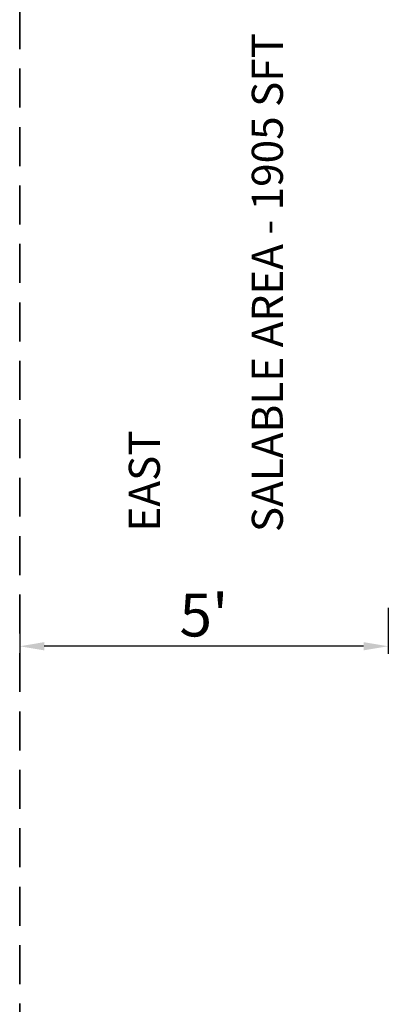
# Model space of a CAD drawing. Units: inches. Extents: x -7 to 1228, y -146 to 1091.
# Tile 2 of 88: x 0 to 60, y 32 to 193. Entities that reach past the tile are written whole.
import ezdxf

# ---------------------------------------------------------------- set-up
doc = ezdxf.new("R2010")
doc.units = ezdxf.units.IN
doc.linetypes.add('DASHED2', pattern=[9.525, 6.35, -3.175])
for name, color, linetype, lineweight in [('A-ANNO-DIMS', 2, 'Continuous', 18), ('A-ANNO-TEXT', 7, 'Continuous', 18), ('C-PROP', 1, 'DASHED2', 35)]:
    doc.layers.add(name, color=color, linetype=linetype, lineweight=lineweight)
doc.styles.get("Standard").update_dxf_attribs({"font": 'arial.ttf'})
doc.dimstyles.new('ISO-25', dxfattribs={"dimtxt": 7, "dimasz": 4, "dimexe": 1.25, "dimexo": 0.625, "dimtad": 1, "dimdec": 1, "dimlunit": 3, "dimtxsty": 'Standard', "dimcen": 2.5, "dimadec": 0, "dimazin": 0, "dimtfac": 1, "dimtdec": 1, "dimtmove": 1, "dimatfit": 3, "dimfxl": 1, "dimarcsym": 0})

# ---------------------------------------------------------------- blocks, each defined once
blk = doc.blocks.new('*D10')
at = {"layer": 'A-ANNO-DIMS', "color": 0, "lineweight": -2, "transparency": 16777216}
for p, q in [((0, 96.81), (0, 89.3)), ((60, 96.81), (60, 89.3)), ((56, 90.55), (4, 90.55))]:
    blk.add_line(p, q, dxfattribs=at)
at = {"layer": 'A-ANNO-DIMS', "color": 0, "transparency": 16777216}
for points in [[(4, 91.22), (4, 89.88), (0, 90.55)], [(56, 91.22), (56, 89.88), (60, 90.55)]]:
    blk.add_solid(points, dxfattribs=at)
at = {"layer": 'Defpoints', "color": 0, "transparency": 16777216}
for p in [(0, 97.43), (60, 97.43), (0, 90.55)]:
    blk.add_point(p, dxfattribs=at)
at = {"layer": 'A-ANNO-DIMS', "color": 0, "transparency": 16777216, "insert": (30, 94.74), "char_height": 7, "attachment_point": 5}
blk.add_mtext("5'", dxfattribs=at)

msp = doc.modelspace()

# ---------------------------------------------------------------- linework, layer by layer
at = {"layer": 'C-PROP'}
msp.add_line((0, 1061), (0, 0), dxfattribs=at)

# ---------------------------------------------------------------- texts
at = {"layer": 'A-ANNO-TEXT', "attachment_point": 1, "rotation": 90}
for s, insert, char_height in [('{SALABLE AREA - 1905 SFT}', (37.8, 109.15), 5.0568), ('EAST', (17.77, 109.24), 5.057)]:
    msp.add_mtext_dynamic_manual_height_columns(s, width=137.2821, gutter_width=25.28, heights=[0], dxfattribs=dict(at, insert=insert, char_height=char_height))

# ---------------------------------------------------------------- dimensions: what is measured, and where the dimension line sits
at = {"layer": 'A-ANNO-DIMS'}
dim = msp.add_linear_dim(base=(0, 90.55), p1=(60, 97.43), p2=(0, 97.43), dimstyle='ISO-25', override={"dimclrd": 0, "dimclre": 0, "dimclrt": 0}, dxfattribs=at)
dim.commit()
dim.dimension.update_dxf_attribs({"geometry": '*D10', "text_midpoint": (30, 94.74)})

doc.saveas('drawing.dxf')
